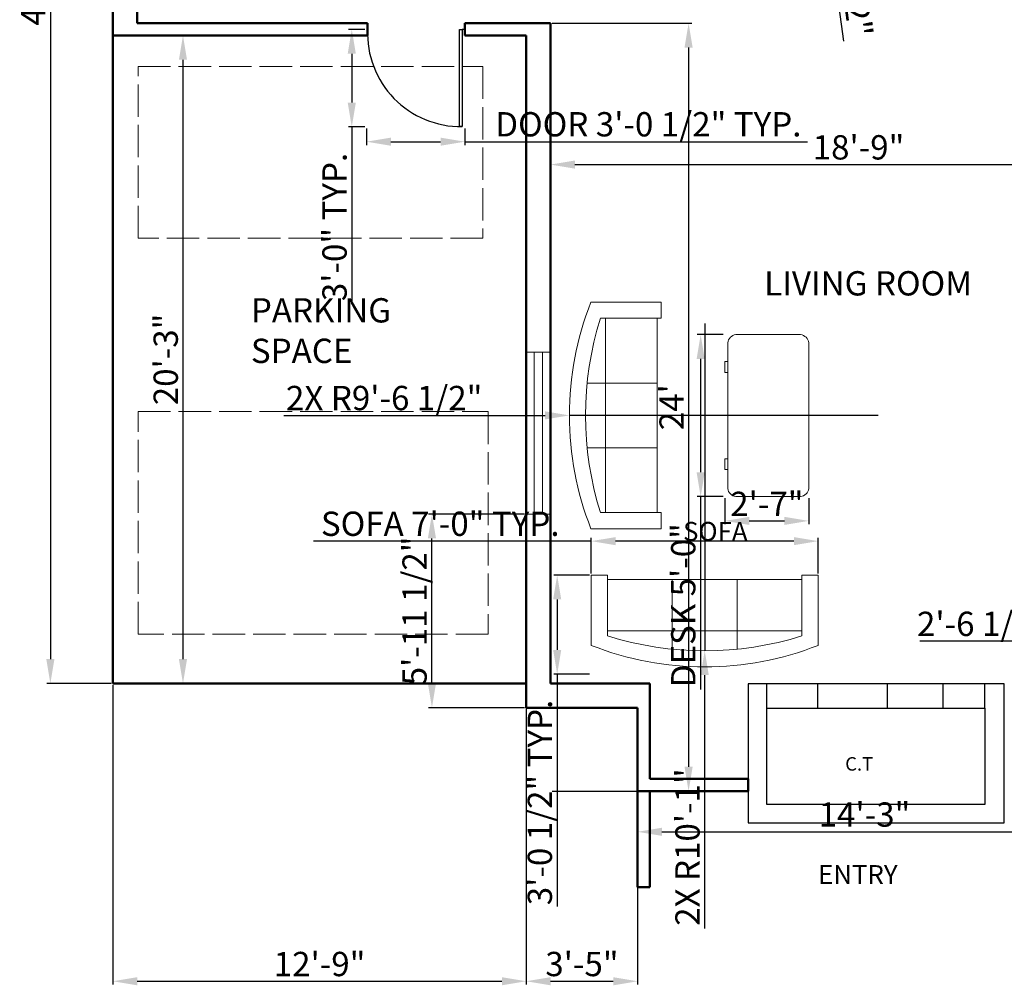
# Model space of a CAD drawing. Units: inches. Extents: x 145135 to 145817, y 90589 to 91373.
# Tile 1 of 4: x 145154 to 145519, y 90615 to 90973. Entities that reach past the tile are written whole.
import ezdxf

# ---------------------------------------------------------------- set-up
doc = ezdxf.new("R2010")
doc.units = ezdxf.units.IN
doc.linetypes.add('ACAD_ISO02W100', pattern=[15, 12, -3])
for name, color, linetype, lineweight in [('A-ANNO-DIMS', 2, 'Continuous', 18), ('A-ANNO-TEXT', 7, 'Continuous', 18), ('A-AREA-IDEN', 7, 'Continuous', 25), ('A-DOOR', 3, 'Continuous', 25), ('A-FLOR-ENTR', 7, 'Continuous', 25), ('A-FLOR-PRKG', 8, 'ACAD_ISO02W100', 13), ('A-FURN', 8, 'Continuous', 18), ('A-GLAZ', 4, 'Continuous', 18), ('A-WALL', 7, 'Continuous', 50)]:
    doc.layers.add(name, color=color, linetype=linetype, lineweight=lineweight)
doc.styles.get("Standard").update_dxf_attribs({"font": 'arial.ttf'})
doc.dimstyles.new('ISO-25', dxfattribs={"dimtxt": 9, "dimasz": 9, "dimexe": 1.25, "dimexo": 0.625, "dimtad": 1, "dimdec": 1, "dimrnd": 9, "dimlunit": 3, "dimtxsty": 'Standard', "dimcen": 2.5, "dimadec": 0, "dimazin": 0, "dimtfac": 1, "dimtdec": 1, "dimtmove": 0, "dimatfit": 3, "dimfxl": 1, "dimarcsym": 0})

# ---------------------------------------------------------------- blocks, each defined once
blk = doc.blocks.new('*D2')
at = {"layer": 'A-ANNO-DIMS', "color": 0, "lineweight": -2, "transparency": 16777216}
for p, q in [((145188.31, 91248.52), (145164.53, 91248.52)), ((145165.78, 91239.52), (145165.78, 90736.31)), ((145188.31, 90727.31), (145164.53, 90727.31))]:
    blk.add_line(p, q, dxfattribs=at)
at = {"layer": 'A-ANNO-DIMS', "color": 0, "transparency": 16777216}
for points in [[(145164.28, 91239.52), (145167.28, 91239.52), (145165.78, 91248.52)], [(145164.28, 90736.31), (145167.28, 90736.31), (145165.78, 90727.31)]]:
    blk.add_solid(points, dxfattribs=at)
at = {"layer": 'Defpoints', "color": 0, "transparency": 16777216}
for p in [(145188.93, 91248.52), (145165.78, 90727.31), (145188.93, 90727.31)]:
    blk.add_point(p, dxfattribs=at)
at = {"layer": 'A-ANNO-DIMS', "color": 0, "transparency": 16777216, "insert": (145160.56, 90987.92), "char_height": 9, "attachment_point": 5, "rotation": 90}
blk.add_mtext('43\'-6"', dxfattribs=at)
blk = doc.blocks.new('*D18')
at = {"layer": 'A-ANNO-DIMS', "color": 0, "lineweight": -2, "transparency": 16777216}
for p, q in [((145350.93, 90971.19), (145350.93, 90918.23)), ((145578.93, 90971.19), (145578.93, 90918.23)), ((145359.93, 90919.48), (145569.93, 90919.48))]:
    blk.add_line(p, q, dxfattribs=at)
at = {"layer": 'A-ANNO-DIMS', "color": 0, "transparency": 16777216}
for points in [[(145359.93, 90920.98), (145359.93, 90917.98), (145350.93, 90919.48)], [(145569.93, 90920.98), (145569.93, 90917.98), (145578.93, 90919.48)]]:
    blk.add_solid(points, dxfattribs=at)
at = {"layer": 'Defpoints', "color": 0, "transparency": 16777216}
for p in [(145350.93, 90971.81), (145578.93, 90971.81), (145578.93, 90919.48)]:
    blk.add_point(p, dxfattribs=at)
at = {"layer": 'A-ANNO-DIMS', "color": 0, "transparency": 16777216, "insert": (145464.93, 90924.7), "char_height": 9, "attachment_point": 5}
blk.add_mtext('18\'-9"', dxfattribs=at)
blk = doc.blocks.new('*D19')
at = {"layer": 'A-ANNO-DIMS', "color": 0, "lineweight": -2, "transparency": 16777216}
for p, q in [((145351.56, 90971.81), (145403.28, 90971.81)), ((145402.03, 90962.81), (145402.03, 90696.41)), ((145351.56, 90687.41), (145403.28, 90687.41))]:
    blk.add_line(p, q, dxfattribs=at)
at = {"layer": 'A-ANNO-DIMS', "color": 0, "transparency": 16777216}
for points in [[(145400.53, 90962.81), (145403.53, 90962.81), (145402.03, 90971.81)], [(145400.53, 90696.41), (145403.53, 90696.41), (145402.03, 90687.41)]]:
    blk.add_solid(points, dxfattribs=at)
at = {"layer": 'Defpoints', "color": 0, "transparency": 16777216}
for p in [(145350.93, 90971.81), (145350.93, 90687.41), (145402.03, 90687.41)]:
    blk.add_point(p, dxfattribs=at)
at = {"layer": 'A-ANNO-DIMS', "color": 0, "transparency": 16777216, "insert": (145396.89, 90829.61), "char_height": 9, "attachment_point": 5, "rotation": 90}
blk.add_mtext("24'", dxfattribs=at)
blk = doc.blocks.new('*D26')
at = {"layer": 'A-ANNO-DIMS', "color": 0, "lineweight": -2, "transparency": 16777216}
for p, q in [((145189.56, 90967.31), (145216.12, 90967.31)), ((145214.87, 90958.31), (145214.87, 90736.31)), ((145189.56, 90727.31), (145216.12, 90727.31))]:
    blk.add_line(p, q, dxfattribs=at)
at = {"layer": 'A-ANNO-DIMS', "color": 0, "transparency": 16777216}
for points in [[(145213.37, 90958.31), (145216.37, 90958.31), (145214.87, 90967.31)], [(145213.37, 90736.31), (145216.37, 90736.31), (145214.87, 90727.31)]]:
    blk.add_solid(points, dxfattribs=at)
at = {"layer": 'Defpoints', "color": 0, "transparency": 16777216}
for p in [(145188.93, 90967.31), (145188.93, 90727.31), (145214.87, 90727.31)]:
    blk.add_point(p, dxfattribs=at)
at = {"layer": 'A-ANNO-DIMS', "color": 0, "transparency": 16777216, "insert": (145209.65, 90847.31), "char_height": 9, "attachment_point": 5, "rotation": 90}
blk.add_mtext('20\'-3"', dxfattribs=at)
blk = doc.blocks.new('*D28')
at = {"layer": 'A-ANNO-DIMS', "color": 0, "lineweight": -2, "transparency": 16777216}
for p, q in [((145383.17, 90686.79), (145383.17, 90671.09)), ((145551.11, 90686.79), (145551.11, 90671.09)), ((145392.17, 90672.34), (145542.11, 90672.34))]:
    blk.add_line(p, q, dxfattribs=at)
at = {"layer": 'A-ANNO-DIMS', "color": 0, "transparency": 16777216}
for points in [[(145392.17, 90673.84), (145392.17, 90670.84), (145383.17, 90672.34)], [(145542.11, 90673.84), (145542.11, 90670.84), (145551.11, 90672.34)]]:
    blk.add_solid(points, dxfattribs=at)
at = {"layer": 'Defpoints', "color": 0, "transparency": 16777216}
for p in [(145383.17, 90687.41), (145551.11, 90687.41), (145551.11, 90672.34)]:
    blk.add_point(p, dxfattribs=at)
at = {"layer": 'A-ANNO-DIMS', "color": 0, "transparency": 16777216, "insert": (145467.14, 90677.57), "char_height": 9, "attachment_point": 5}
blk.add_mtext('14\'-3"', dxfattribs=at)
blk = doc.blocks.new('Sofa - Roundback 7 ft.')
for p, q in [((-12.00002, -32.4421), (-12.00003, -6.5971)), ((11.99997, -32.4421), (11.99998, -6.5971)), ((-36.000027, -34), (-36.000027, -11.4696)), ((-35.999844, -13.3819), (35.9998, -13.3819)), ((35.99998, -34), (35.99998, -11.4696)), ((-36.000027, -32.4421), (35.99998, -32.4421))]:
    blk.add_line(p, q)
for points in [[(-36.000027, -34), (-42.000027, -34), (-42.000027, -8)], [(41.99998, -8), (41.99998, -34), (35.99998, -34)]]:
    blk.add_lwpolyline(points)
for centre, radius, start, end in [((0, -114.25), 114.25, 68.43141, 111.5686), ((-0.00001, -127.1968), 121.1968, 72.72033, 107.2797)]:
    blk.add_arc(centre, radius, start, end)
blk = doc.blocks.new('Desk - 30 x 60 in.')
for p, q in [((-26.999995, 0), (26.999995, 0)), ((-29.999995, -27), (-29.999995, -3)), ((29.999995, -3), (29.999995, -27)), ((26.999995, -30), (-26.999995, -30)), ((-20.000005, -30), (-20.000005, -31)), ((-20.000005, -31), (-16.000005, -31)), ((-16.000005, -31), (-16.000005, -30)), ((15.999995, -31), (15.999995, -30)), ((19.999995, -31), (15.999995, -31)), ((19.999995, -30), (19.999995, -31))]:
    blk.add_line(p, q)
for centre, start, end in [((-26.499995, -3.5), 98.1301, 171.8699), ((26.499995, -3.5), 8.130102, 81.8699), ((-26.499995, -26.5), 188.1301, 261.8699), ((26.499995, -26.5), 278.1301, 351.8699)]:
    blk.add_arc(centre, 3.535534, start, end)
blk = doc.blocks.new('WIN-60IN')
for p, q in [((0, 9), (0, 0)), ((60, 9), (60, 0)), ((60, 6), (0, 6)), ((60, 3), (0, 3))]:
    blk.add_line(p, q)
blk = doc.blocks.new('DOOR-SWING-36IN')
for p, q in [((0, 36.03), (0, 35.03)), ((0, 35.03), (36, 35.03)), ((0, 34.03), (0, 35.03)), ((36, 34.03), (0, 34.03)), ((36, 35.03), (36, 34.03))]:
    blk.add_line(p, q)
blk.add_arc((1.47, 34.53), 34.53, 267.5565, 0.8296)
blk = doc.blocks.new('*D44')
at = {"layer": 'A-ANNO-DIMS', "color": 0, "lineweight": -2, "transparency": 16777216}
for p, q in [((145366, 90780), (145263.21, 90780)), ((145366, 90768.03), (145366, 90781.25)), ((145441, 90780), (145375, 90780)), ((145450, 90768.03), (145450, 90781.25))]:
    blk.add_line(p, q, dxfattribs=at)
at = {"layer": 'A-ANNO-DIMS', "color": 0, "transparency": 16777216}
for points in [[(145375, 90781.5), (145375, 90778.5), (145366, 90780)], [(145441, 90781.5), (145441, 90778.5), (145450, 90780)]]:
    blk.add_solid(points, dxfattribs=at)
at = {"layer": 'Defpoints', "color": 0, "transparency": 16777216}
for p in [(145366, 90780), (145366, 90767.4), (145450, 90767.4)]:
    blk.add_point(p, dxfattribs=at)
at = {"layer": 'A-ANNO-DIMS', "color": 0, "transparency": 16777216, "insert": (145310.1, 90785.28), "char_height": 9, "attachment_point": 5}
blk.add_mtext('SOFA 7\'-0" TYP.', dxfattribs=at)
blk = doc.blocks.new('*D45')
at = {"layer": 'A-ANNO-DIMS', "color": 0, "lineweight": -2, "transparency": 16777216}
for p, q in [((145365.37, 90767.4), (145352.15, 90767.4)), ((145353.4, 90758.4), (145353.4, 90739.74)), ((145365.37, 90730.74), (145352.15, 90730.74)), ((145353.4, 90730.74), (145353.4, 90644.66))]:
    blk.add_line(p, q, dxfattribs=at)
at = {"layer": 'A-ANNO-DIMS', "color": 0, "transparency": 16777216}
for points in [[(145351.9, 90758.4), (145354.9, 90758.4), (145353.4, 90767.4)], [(145351.9, 90739.74), (145354.9, 90739.74), (145353.4, 90730.74)]]:
    blk.add_solid(points, dxfattribs=at)
at = {"layer": 'Defpoints', "color": 0, "transparency": 16777216}
for p in [(145366, 90767.4), (145353.4, 90730.74), (145366, 90730.74)]:
    blk.add_point(p, dxfattribs=at)
at = {"layer": 'A-ANNO-DIMS', "color": 0, "transparency": 16777216, "insert": (145348.12, 90683.2), "char_height": 9, "attachment_point": 5, "rotation": 90}
blk.add_mtext('3\'-0 1/2" TYP.', dxfattribs=at)
blk = doc.blocks.new('*D48')
at = {"layer": 'A-ANNO-DIMS', "color": 0, "lineweight": -2, "transparency": 16777216}
for p, q in [((145282.82, 90932.8), (145282.82, 90926.71)), ((145319.22, 90932.8), (145319.22, 90926.71)), ((145291.82, 90927.96), (145310.22, 90927.96)), ((145319.22, 90927.96), (145446.07, 90927.96))]:
    blk.add_line(p, q, dxfattribs=at)
at = {"layer": 'A-ANNO-DIMS', "color": 0, "transparency": 16777216}
for points in [[(145291.82, 90929.46), (145291.82, 90926.46), (145282.82, 90927.96)], [(145310.22, 90929.46), (145310.22, 90926.46), (145319.22, 90927.96)]]:
    blk.add_solid(points, dxfattribs=at)
at = {"layer": 'Defpoints', "color": 0, "transparency": 16777216}
for p in [(145282.82, 90933.43), (145319.22, 90933.43), (145319.22, 90927.96)]:
    blk.add_point(p, dxfattribs=at)
at = {"layer": 'A-ANNO-DIMS', "color": 0, "transparency": 16777216, "insert": (145387.14, 90933.25), "char_height": 9, "attachment_point": 5}
blk.add_mtext('DOOR 3\'-0 1/2" TYP.', dxfattribs=at)
blk = doc.blocks.new('*D49')
at = {"layer": 'A-ANNO-DIMS', "color": 0, "lineweight": -2, "transparency": 16777216}
for p, q in [((145282.19, 90969.56), (145276.11, 90969.56)), ((145277.36, 90960.56), (145277.36, 90942.43)), ((145282.19, 90933.43), (145276.11, 90933.43)), ((145277.36, 90933.43), (145277.36, 90868.32))]:
    blk.add_line(p, q, dxfattribs=at)
at = {"layer": 'A-ANNO-DIMS', "color": 0, "transparency": 16777216}
for points in [[(145275.86, 90960.56), (145278.86, 90960.56), (145277.36, 90969.56)], [(145275.86, 90942.43), (145278.86, 90942.43), (145277.36, 90933.43)]]:
    blk.add_solid(points, dxfattribs=at)
at = {"layer": 'Defpoints', "color": 0, "transparency": 16777216}
for p in [(145282.82, 90969.56), (145277.36, 90933.43), (145282.82, 90933.43)]:
    blk.add_point(p, dxfattribs=at)
at = {"layer": 'A-ANNO-DIMS', "color": 0, "transparency": 16777216, "insert": (145272.13, 90896.37), "char_height": 9, "attachment_point": 5, "rotation": 90}
blk.add_mtext('3\'-0" TYP.', dxfattribs=at)
blk = doc.blocks.new('*D54')
at = {"layer": 'A-ANNO-DIMS', "color": 0, "lineweight": -2, "transparency": 16777216}
for p, q in [((145414.88, 90856.5), (145405.25, 90856.5)), ((145406.5, 90847.5), (145406.5, 90805.5)), ((145414.88, 90796.5), (145405.25, 90796.5)), ((145406.5, 90796.5), (145406.5, 90725.04))]:
    blk.add_line(p, q, dxfattribs=at)
at = {"layer": 'A-ANNO-DIMS', "color": 0, "transparency": 16777216}
for points in [[(145405, 90847.5), (145408, 90847.5), (145406.5, 90856.5)], [(145405, 90805.5), (145408, 90805.5), (145406.5, 90796.5)]]:
    blk.add_solid(points, dxfattribs=at)
at = {"layer": 'Defpoints', "color": 0, "transparency": 16777216}
for p in [(145415.5, 90856.5), (145406.5, 90796.5), (145415.5, 90796.5)]:
    blk.add_point(p, dxfattribs=at)
at = {"layer": 'A-ANNO-DIMS', "color": 0, "transparency": 16777216, "insert": (145401.22, 90756.27), "char_height": 9, "attachment_point": 5, "rotation": 90}
blk.add_mtext('DESK 5\'-0"', dxfattribs=at)
blk = doc.blocks.new('*D55')
at = {"layer": 'A-ANNO-DIMS', "color": 0, "lineweight": -2, "transparency": 16777216}
for p, q in [((145415.5, 90795.87), (145415.5, 90786.25)), ((145446.5, 90795.87), (145446.5, 90786.25)), ((145424.5, 90787.5), (145437.5, 90787.5))]:
    blk.add_line(p, q, dxfattribs=at)
at = {"layer": 'A-ANNO-DIMS', "color": 0, "transparency": 16777216}
for points in [[(145424.5, 90789), (145424.5, 90786), (145415.5, 90787.5)], [(145437.5, 90789), (145437.5, 90786), (145446.5, 90787.5)]]:
    blk.add_solid(points, dxfattribs=at)
at = {"layer": 'Defpoints', "color": 0, "transparency": 16777216}
for p in [(145415.5, 90796.5), (145446.5, 90796.5), (145446.5, 90787.5)]:
    blk.add_point(p, dxfattribs=at)
at = {"layer": 'A-ANNO-DIMS', "color": 0, "transparency": 16777216, "insert": (145431, 90792.64), "char_height": 9, "attachment_point": 5}
blk.add_mtext('2\'-7"', dxfattribs=at)
blk = doc.blocks.new('*D56')
at = {"layer": 'A-ANNO-DIMS', "color": 0, "lineweight": -2, "transparency": 16777216}
for p, q in [((145188.93, 90726.69), (145188.93, 90615.73)), ((145341.93, 90726.69), (145341.93, 90615.73)), ((145197.93, 90616.98), (145332.93, 90616.98))]:
    blk.add_line(p, q, dxfattribs=at)
at = {"layer": 'A-ANNO-DIMS', "color": 0, "transparency": 16777216}
for points in [[(145197.93, 90618.48), (145197.93, 90615.48), (145188.93, 90616.98)], [(145332.93, 90618.48), (145332.93, 90615.48), (145341.93, 90616.98)]]:
    blk.add_solid(points, dxfattribs=at)
at = {"layer": 'Defpoints', "color": 0, "transparency": 16777216}
for p in [(145188.93, 90727.31), (145341.93, 90727.31), (145341.93, 90616.98)]:
    blk.add_point(p, dxfattribs=at)
at = {"layer": 'A-ANNO-DIMS', "color": 0, "transparency": 16777216, "insert": (145265.43, 90622.2), "char_height": 9, "attachment_point": 5}
blk.add_mtext('12\'-9"', dxfattribs=at)
blk = doc.blocks.new('*D63')
at = {"layer": 'A-ANNO-DIMS', "color": 0, "lineweight": -2, "transparency": 16777216}
for p, q in [((145341.31, 90790), (145305.78, 90790)), ((145307.03, 90727.31), (145307.03, 90781)), ((145341.31, 90718.31), (145305.78, 90718.31))]:
    blk.add_line(p, q, dxfattribs=at)
at = {"layer": 'A-ANNO-DIMS', "color": 0, "transparency": 16777216}
for points in [[(145305.53, 90781), (145308.53, 90781), (145307.03, 90790)], [(145305.53, 90727.31), (145308.53, 90727.31), (145307.03, 90718.31)]]:
    blk.add_solid(points, dxfattribs=at)
at = {"layer": 'Defpoints', "color": 0, "transparency": 16777216}
for p in [(145307.03, 90790), (145341.93, 90790), (145341.93, 90718.31)]:
    blk.add_point(p, dxfattribs=at)
at = {"layer": 'A-ANNO-DIMS', "color": 0, "transparency": 16777216, "insert": (145301.76, 90754.16), "char_height": 9, "attachment_point": 5, "rotation": 90}
blk.add_mtext('5\'-11 1/2"', dxfattribs=at)
blk = doc.blocks.new('*D68')
at = {"layer": 'A-ANNO-DIMS', "color": 0, "lineweight": -2, "transparency": 16777216}
for p, q in [((145341.93, 90717.69), (145341.93, 90615.73)), ((145383.17, 90717.69), (145383.17, 90615.73)), ((145350.93, 90616.98), (145374.17, 90616.98))]:
    blk.add_line(p, q, dxfattribs=at)
at = {"layer": 'A-ANNO-DIMS', "color": 0, "transparency": 16777216}
for points in [[(145350.93, 90618.48), (145350.93, 90615.48), (145341.93, 90616.98)], [(145374.17, 90618.48), (145374.17, 90615.48), (145383.17, 90616.98)]]:
    blk.add_solid(points, dxfattribs=at)
at = {"layer": 'Defpoints', "color": 0, "transparency": 16777216}
for p in [(145341.93, 90718.31), (145383.17, 90718.31), (145383.17, 90616.98)]:
    blk.add_point(p, dxfattribs=at)
at = {"layer": 'A-ANNO-DIMS', "color": 0, "transparency": 16777216, "insert": (145362.55, 90622.2), "char_height": 9, "attachment_point": 5}
blk.add_mtext('3\'-5"', dxfattribs=at)
blk = doc.blocks.new('*D72')
at = {"layer": 'A-ANNO-DIMS', "color": 0, "lineweight": -2, "transparency": 16777216}
for p, q in [((145542.89, 90777.19), (145542.89, 90741.67)), ((145573.55, 90777.19), (145573.55, 90741.67)), ((145542.89, 90742.92), (145487.59, 90742.92)), ((145564.55, 90742.92), (145551.89, 90742.92))]:
    blk.add_line(p, q, dxfattribs=at)
at = {"layer": 'A-ANNO-DIMS', "color": 0, "transparency": 16777216}
for points in [[(145551.89, 90744.42), (145551.89, 90741.42), (145542.89, 90742.92)], [(145564.55, 90744.42), (145564.55, 90741.42), (145573.55, 90742.92)]]:
    blk.add_solid(points, dxfattribs=at)
at = {"layer": 'Defpoints', "color": 0, "transparency": 16777216}
for p in [(145542.89, 90777.82), (145573.55, 90777.82), (145542.89, 90742.92)]:
    blk.add_point(p, dxfattribs=at)
at = {"layer": 'A-ANNO-DIMS', "color": 0, "transparency": 16777216, "insert": (145510.74, 90748.2), "char_height": 9, "attachment_point": 5}
blk.add_mtext('2\'-6 1/2"', dxfattribs=at)
blk = doc.blocks.new('*D81')
at = {"layer": 'A-ANNO-DIMS', "color": 0, "lineweight": -2, "transparency": 16777216}
for p, q in [((145408, 90860.6), (145408, 90739.4)), ((145408, 90636.55), (145408, 90730.4))]:
    blk.add_line(p, q, dxfattribs=at)
at = {"layer": 'A-ANNO-DIMS', "color": 0, "transparency": 16777216}
blk.add_solid([(145406.5, 90730.4), (145409.5, 90730.4), (145408, 90739.4)], dxfattribs=at)
at = {"layer": 'Defpoints', "color": 0, "transparency": 16777216}
for p in [(145408, 90860.6), (145408, 90739.4)]:
    blk.add_point(p, dxfattribs=at)
at = {"layer": 'A-ANNO-DIMS', "color": 0, "transparency": 16777216, "insert": (145402.78, 90666.68), "char_height": 9, "attachment_point": 5, "rotation": 90}
blk.add_mtext('2X R10\'-1"', dxfattribs=at)
blk = doc.blocks.new('*D82')
at = {"layer": 'A-ANNO-DIMS', "color": 0, "lineweight": -2, "transparency": 16777216}
for p, q in [((145252.22, 90826.58), (145348.9, 90826.58)), ((145472.15, 90826.58), (145357.9, 90826.58))]:
    blk.add_line(p, q, dxfattribs=at)
at = {"layer": 'A-ANNO-DIMS', "color": 0, "transparency": 16777216}
blk.add_solid([(145348.9, 90828.08), (145348.9, 90825.08), (145357.9, 90826.58)], dxfattribs=at)
at = {"layer": 'Defpoints', "color": 0, "transparency": 16777216}
for p in [(145357.9, 90826.58), (145472.15, 90826.58)]:
    blk.add_point(p, dxfattribs=at)
at = {"layer": 'A-ANNO-DIMS', "color": 0, "transparency": 16777216, "insert": (145289.35, 90831.85), "char_height": 9, "attachment_point": 5, "rotation": 359.9999}
blk.add_mtext('2X R9\'-6 1/2"', dxfattribs=at)
blk = doc.blocks.new('*D84')
at = {"layer": 'A-ANNO-DIMS', "color": 0, "lineweight": -2, "transparency": 16777216}
for p, q in [((145444.75, 91074.95), (145446.26, 91063.73)), ((145459.51, 90965.16), (145447.46, 91054.81))]:
    blk.add_line(p, q, dxfattribs=at)
at = {"layer": 'A-ANNO-DIMS', "color": 0, "transparency": 16777216}
blk.add_solid([(145448.95, 91055.01), (145445.97, 91054.61), (145446.26, 91063.73)], dxfattribs=at)
at = {"layer": 'Defpoints', "color": 0, "transparency": 16777216}
for p in [(145444.75, 91074.95), (145446.26, 91063.73)]:
    blk.add_point(p, dxfattribs=at)
at = {"layer": 'A-ANNO-DIMS', "color": 0, "transparency": 16777216, "insert": (145459.32, 91006.23), "char_height": 9, "attachment_point": 5, "rotation": 277.655}
blk.add_mtext('4X R0\'-11 1/2"', dxfattribs=at)

msp = doc.modelspace()

# ---------------------------------------------------------------- linework, layer by layer
at = {"layer": 'A-FLOR-ENTR'}
for p, q in [((145431, 90718.1), (145431, 90727.1)), ((145449.85, 90718.1), (145449.85, 90727.1)), ((145475.65, 90718.1), (145475.65, 90727.1)), ((145496.22, 90718.1), (145496.22, 90727.1)), ((145511.74, 90718.1), (145511.74, 90727.1))]:
    msp.add_line(p, q, dxfattribs=at)
for points in [[(145424.03, 90675.63), (145518.85, 90675.63), (145518.85, 90727.1), (145424.03, 90727.1)], [(145431, 90718.1), (145511.74, 90718.1), (145511.74, 90682.43), (145431, 90682.43)]]:
    msp.add_lwpolyline(points, close=True, dxfattribs=at)
at = {"layer": 'A-FLOR-PRKG'}
for points in [[(145198.25, 90955.78), (145325.91, 90955.78), (145325.91, 90892.19), (145198.25, 90892.19)], [(145198.25, 90827.98), (145327.83, 90827.98), (145327.83, 90745.51), (145198.25, 90745.51)]]:
    msp.add_lwpolyline(points, close=True, dxfattribs=at)
at = {"layer": 'A-WALL'}
for p, q in [((145188.93, 90727.31), (145188.93, 91248.52)), ((145197.93, 90971.81), (145197.93, 91010.02)), ((145283.22, 90971.81), (145197.93, 90971.81)), ((145283.22, 90971.81), (145283.22, 90967.31)), ((145341.93, 90971.81), (145319.22, 90971.81)), ((145319.22, 90971.81), (145350.93, 90971.81)), ((145319.22, 90971.81), (145319.22, 90967.31)), ((145350.93, 90727.31), (145350.93, 90971.81)), ((145197.93, 90967.31), (145188.93, 90967.31)), ((145283.22, 90967.31), (145197.93, 90967.31)), ((145341.93, 90967.31), (145319.22, 90967.31)), ((145341.93, 90718.31), (145341.93, 90967.31)), ((145197.93, 90727.31), (145188.93, 90727.31)), ((145341.93, 90727.31), (145197.93, 90727.31)), ((145350.93, 90727.31), (145387.67, 90727.31)), ((145387.67, 90727.31), (145387.67, 90691.91)), ((145341.93, 90718.31), (145383.17, 90718.31)), ((145383.17, 90718.31), (145383.17, 90687.41)), ((145387.67, 90691.91), (145424.03, 90691.91)), ((145424.03, 90691.91), (145424.03, 90687.41)), ((145383.17, 90687.41), (145424.03, 90687.41)), ((145383.17, 90687.41), (145383.17, 90651.88)), ((145387.67, 90687.41), (145387.67, 90651.88)), ((145383.17, 90651.88), (145387.67, 90651.88))]:
    msp.add_line(p, q, dxfattribs=at)

# ---------------------------------------------------------------- block references
at = {"layer": 'A-DOOR', "rotation": 270.0000000001312}
msp.add_blockref('DOOR-SWING-36IN', (145283.19, 90969.56), dxfattribs=at)
at = {"layer": 'A-FURN'}
for name, p, rotation in [('Sofa - Roundback 7 ft.', (145357.9, 90826.58), 89.99999999999999), ('Desk - 30 x 60 in.', (145446.5, 90826.5), 270), ('Sofa - Roundback 7 ft.', (145408, 90733.4), 180)]:
    msp.add_blockref(name, p, dxfattribs=dict(at, rotation=rotation))
at = {"layer": 'A-GLAZ', "rotation": 90.00000000010874}
msp.add_blockref('WIN-60IN', (145350.93, 90790), dxfattribs=at)

# ---------------------------------------------------------------- texts
at = {"layer": 'A-ANNO-TEXT', "attachment_point": 1}
for s, width, insert, char_height in [('SOFA', 520, (145400, 90787.12), 7), ('C.T', 20.1144, (145460, 90700), 5)]:
    msp.add_mtext_dynamic_manual_height_columns(s, width=width, gutter_width=12.5, heights=[0], dxfattribs=dict(at, insert=insert, char_height=char_height))
at = {"layer": 'A-AREA-IDEN', "attachment_point": 1}
for s, width, insert, char_height in [('LIVING ROOM', 90, (145430, 90880), 9), ('PARKING \\PSPACE', 90, (145240, 90870), 9), ('ENTRY', 520, (145450, 90660), 7)]:
    msp.add_mtext_dynamic_manual_height_columns(s, width=width, gutter_width=12.5, heights=[0], dxfattribs=dict(at, insert=insert, char_height=char_height))

# ---------------------------------------------------------------- dimensions: what is measured, and where the dimension line sits
at = {"layer": 'A-ANNO-DIMS'}
for base, p1, p2, angle, override, picture, middle in [((145165.78, 90727.31), (145188.93, 91248.52), (145188.93, 90727.31), 90, {"dimclrd": 0, "dimclre": 0, "dimclrt": 0}, '*D2', (145160.56, 90987.92)), ((145402.03, 90687.41), (145350.93, 90971.81), (145350.93, 90687.41), 90, {"dimclrd": 0, "dimclre": 0, "dimclrt": 0}, '*D19', (145396.89, 90829.61)), ((145214.87, 90727.31), (145188.93, 90967.31), (145188.93, 90727.31), 90, {"dimclrd": 0, "dimclre": 0, "dimclrt": 0}, '*D26', (145209.65, 90847.31)), ((145307.03, 90790), (145341.93, 90718.31), (145341.93, 90790), 90, {"dimdec": 1, "dimlfac": 1, "dimrnd": 0, "dimzin": 1, "dimdsep": 46, "dimlunit": 4, "dimfrac": 2}, '*D63', (145301.76, 90754.16)), ((145542.89, 90742.92), (145573.55, 90777.82), (145542.89, 90777.82), 180, {"dimdec": 1, "dimlfac": 1, "dimrnd": 0, "dimzin": 1, "dimdsep": 46, "dimlunit": 4, "dimfrac": 2}, '*D72', (145510.74, 90748.2))]:
    dim = msp.add_linear_dim(base=base, p1=p1, p2=p2, angle=angle, dimstyle='ISO-25', override=override, dxfattribs=at)
    dim.commit()
    dim.dimension.update_dxf_attribs({"geometry": picture, "text_midpoint": middle})
dim = msp.add_radius_dim(center=(145444.75, 91074.95), mpoint=(145446.26, 91063.73), text='4X <>', dimstyle='ISO-25', override={"dimdec": 1, "dimlfac": 1, "dimrnd": 0, "dimzin": 1, "dimdsep": 46, "dimlunit": 4, "dimfrac": 2}, dxfattribs=at)
dim.commit()
dim.dimension.update_dxf_attribs({"geometry": '*D84', "text_midpoint": (145459.32, 91006.23)})
for base, p1, p2, angle, text, picture, middle in [((145277.36, 90933.43), (145282.82, 90969.56), (145282.82, 90933.43), 270, '<> TYP.', '*D49', (145272.13, 90896.37)), ((145319.22, 90927.96), (145282.82, 90933.43), (145319.22, 90933.43), 0, 'DOOR <> TYP.', '*D48', (145387.14, 90933.25)), ((145406.5, 90796.5), (145415.5, 90856.5), (145415.5, 90796.5), 270, 'DESK <>', '*D54', (145401.22, 90756.27)), ((145366, 90780), (145450, 90767.4), (145366, 90767.4), 180, 'SOFA <> TYP.', '*D44', (145310.1, 90785.28)), ((145353.4, 90730.74), (145366, 90767.4), (145366, 90730.74), 270, '<> TYP.', '*D45', (145348.12, 90683.2))]:
    dim = msp.add_linear_dim(base=base, p1=p1, p2=p2, angle=angle, text=text, dimstyle='ISO-25', override={"dimdec": 1, "dimlfac": 1, "dimrnd": 0, "dimzin": 1, "dimdsep": 46, "dimlunit": 4, "dimfrac": 2}, dxfattribs=at)
    dim.commit()
    dim.dimension.update_dxf_attribs({"geometry": picture, "text_midpoint": middle})
for base, p1, p2, override, picture, middle in [((145578.93, 90919.48), (145350.93, 90971.81), (145578.93, 90971.81), {"dimclrd": 0, "dimclre": 0, "dimclrt": 0}, '*D18', (145464.93, 90924.7)), ((145446.5, 90787.5), (145415.5, 90796.5), (145446.5, 90796.5), {"dimdec": 1, "dimlfac": 1, "dimrnd": 0, "dimzin": 1, "dimdsep": 46, "dimlunit": 4, "dimfrac": 2}, '*D55', (145431, 90792.64)), ((145341.93, 90616.98), (145188.93, 90727.31), (145341.93, 90727.31), {"dimdec": 1, "dimlfac": 1, "dimrnd": 0, "dimzin": 1, "dimdsep": 46, "dimlunit": 4, "dimfrac": 2}, '*D56', (145265.43, 90622.2)), ((145383.17, 90616.98), (145341.93, 90718.31), (145383.17, 90718.31), {"dimdec": 1, "dimlfac": 1, "dimrnd": 0, "dimzin": 1, "dimdsep": 46, "dimlunit": 4, "dimfrac": 2}, '*D68', (145362.55, 90622.2)), ((145551.11, 90672.34), (145383.17, 90687.41), (145551.11, 90687.41), {"dimclrd": 0, "dimclre": 0, "dimclrt": 0}, '*D28', (145467.14, 90677.57))]:
    dim = msp.add_linear_dim(base=base, p1=p1, p2=p2, dimstyle='ISO-25', override=override, dxfattribs=at)
    dim.commit()
    dim.dimension.update_dxf_attribs({"geometry": picture, "text_midpoint": middle})
for center, mpoint, picture, middle in [((145408, 90860.6), (145408, 90739.4), '*D81', (145408, 90666.68)), ((145472.147043, 90826.575866), (145357.897043, 90826.576), '*D82', (145289.347043, 90826.5760804))]:
    dim = msp.add_radius_dim(center=center, mpoint=mpoint, text='2X <>', dimstyle='ISO-25', override={"dimdec": 1, "dimlfac": 1, "dimrnd": 0, "dimzin": 1, "dimdsep": 46, "dimlunit": 4, "dimfrac": 2}, dxfattribs=at)
    dim.commit()
    dim.dimension.update_dxf_attribs({"geometry": picture, "text_midpoint": middle, "dimtype": 164})

doc.saveas('drawing.dxf')
